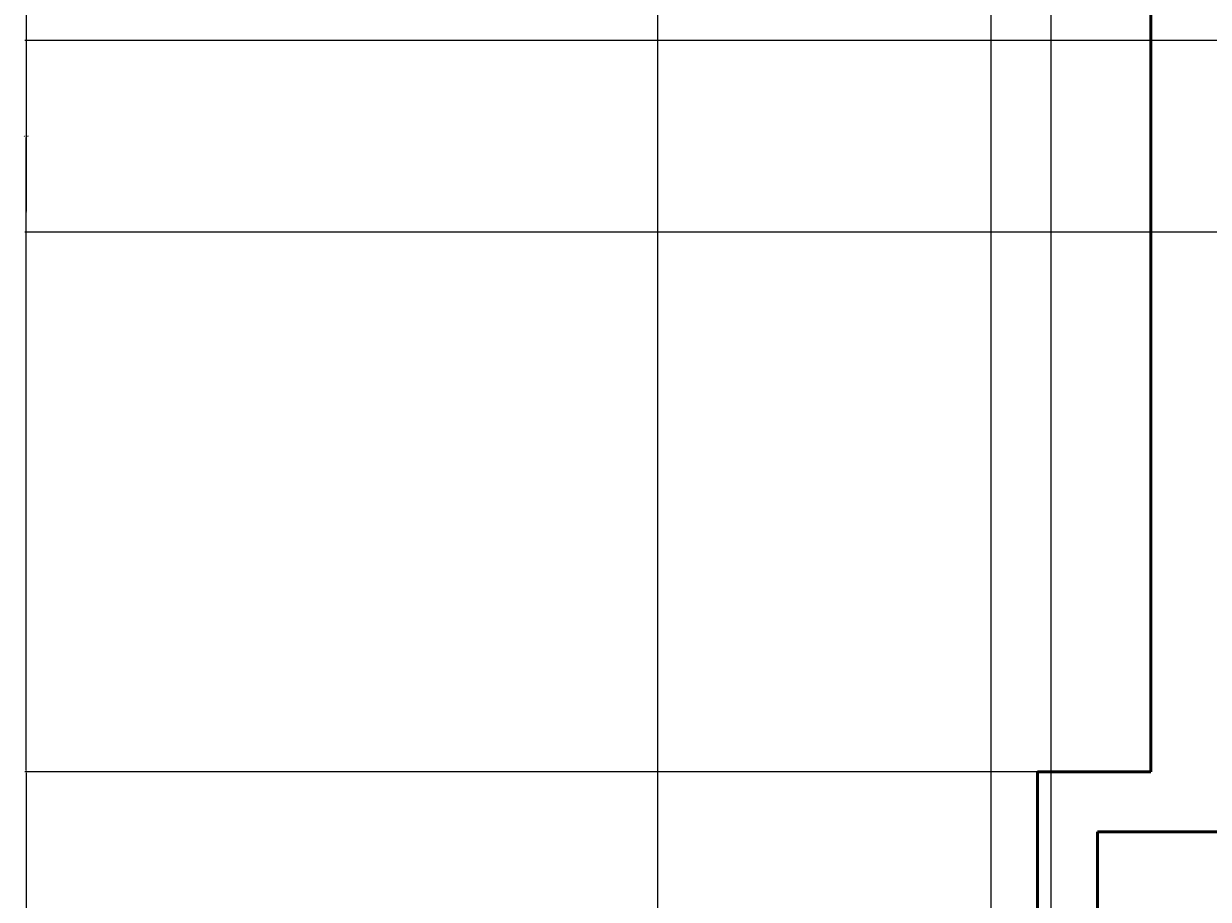
# Model space of a CAD drawing. Units: inches. Extents: x 5375 to 6084, y 16106 to 17259.
# Tile 18 of 32: x 5375 to 5553, y 16680 to 16812. Entities that reach past the tile are written whole.
import ezdxf

# ---------------------------------------------------------------- set-up
doc = ezdxf.new("R2010")
doc.units = ezdxf.units.IN
doc.layers.add('A-ANNO-DIMS', color=2, linetype='Continuous', lineweight=18)
doc.layers.add('WALL', color=6, linetype='Continuous', lineweight=50)
doc.styles.get("Standard").update_dxf_attribs({"font": 'arial.ttf'})
doc.dimstyles.get("Standard").update_dxf_attribs({"dimtxt": 0.18, "dimasz": 0.18, "dimexe": 0.18, "dimexo": 0.0625, "dimgap": 0.09, "dimtad": 0, "dimtih": 1, "dimtoh": 1, "dimdec": 4, "dimzin": 0, "dimdsep": 46, "dimtxsty": 'Standard', "dimcen": 0.09, "dimadec": 0, "dimazin": 0, "dimtfac": 1, "dimtdec": 4, "dimtofl": 0, "dimtmove": 0, "dimatfit": 3, "dimfxl": 1, "dimtolj": 1, "dimtzin": 0, "dimarcsym": 0})

# ---------------------------------------------------------------- blocks, each defined once
blk = doc.blocks.new('*D35')
at = {"layer": 'A-ANNO-DIMS', "color": 0, "lineweight": -2, "transparency": 16777216}
for p, q in [((5527.56, 16699.58), (5375.56, 16699.58)), ((5375.74, 16699.4), (5375.74, 16651.76)), ((5375.74, 16603.76), (5375.74, 16651.4)), ((5527.56, 16603.58), (5375.56, 16603.58))]:
    blk.add_line(p, q, dxfattribs=at)
at = {"layer": 'A-ANNO-DIMS', "color": 0, "transparency": 16777216}
for points in [[(5375.71, 16699.4), (5375.77, 16699.4), (5375.74, 16699.58)], [(5375.71, 16603.76), (5375.77, 16603.76), (5375.74, 16603.58)]]:
    blk.add_solid(points, dxfattribs=at)
at = {"layer": 'Defpoints', "color": 0, "transparency": 16777216}
for p in [(5375.74, 16699.58), (5527.62, 16699.58), (5527.62, 16603.58)]:
    blk.add_point(p, dxfattribs=at)
at = {"layer": 'A-ANNO-DIMS', "color": 0, "transparency": 16777216, "insert": (5375.74, 16651.58), "char_height": 0.18, "attachment_point": 5}
blk.add_mtext('\\A1;96', dxfattribs=at)
blk = doc.blocks.new('*D36')
at = {"layer": 'A-ANNO-DIMS', "color": 0, "lineweight": -2, "transparency": 16777216}
for p, q in [((5544.56, 16867.58), (5375.56, 16867.58)), ((5375.74, 16867.4), (5375.74, 16783.76)), ((5375.74, 16699.76), (5375.74, 16783.4)), ((5544.56, 16699.58), (5375.56, 16699.58))]:
    blk.add_line(p, q, dxfattribs=at)
at = {"layer": 'A-ANNO-DIMS', "color": 0, "transparency": 16777216}
for points in [[(5375.71, 16867.4), (5375.77, 16867.4), (5375.74, 16867.58)], [(5375.71, 16699.76), (5375.77, 16699.76), (5375.74, 16699.58)]]:
    blk.add_solid(points, dxfattribs=at)
at = {"layer": 'Defpoints', "color": 0, "transparency": 16777216}
for p in [(5375.74, 16867.58), (5544.62, 16867.58), (5544.62, 16699.58)]:
    blk.add_point(p, dxfattribs=at)
at = {"layer": 'A-ANNO-DIMS', "color": 0, "transparency": 16777216, "insert": (5375.74, 16783.58), "char_height": 0.18, "attachment_point": 5}
blk.add_mtext('\\A1;168', dxfattribs=at)
blk = doc.blocks.new('*D40')
at = {"layer": 'A-ANNO-DIMS', "color": 0, "lineweight": -2, "transparency": 16777216}
for p, q in [((5529.62, 16876.52), (5529.62, 16106.48)), ((5520.62, 16867.52), (5520.62, 16106.48)), ((5520.8, 16106.66), (5524.97, 16106.66)), ((5529.44, 16106.66), (5525.27, 16106.66))]:
    blk.add_line(p, q, dxfattribs=at)
at = {"layer": 'A-ANNO-DIMS', "color": 0, "transparency": 16777216}
for points in [[(5520.8, 16106.69), (5520.8, 16106.63), (5520.62, 16106.66)], [(5529.44, 16106.69), (5529.44, 16106.63), (5529.62, 16106.66)]]:
    blk.add_solid(points, dxfattribs=at)
at = {"layer": 'Defpoints', "color": 0, "transparency": 16777216}
for p in [(5529.62, 16876.58), (5520.62, 16867.58), (5529.62, 16106.66)]:
    blk.add_point(p, dxfattribs=at)
at = {"layer": 'A-ANNO-DIMS', "color": 0, "transparency": 16777216, "insert": (5525.12, 16106.66), "char_height": 0.18, "attachment_point": 5}
blk.add_mtext('\\A1;9', dxfattribs=at)
blk = doc.blocks.new('*D43')
at = {"layer": 'A-ANNO-DIMS', "color": 0, "lineweight": -2, "transparency": 16777216}
for p, q in [((5826.06, 16809.37), (5375.56, 16809.37)), ((5375.74, 16809.19), (5375.74, 16795.15)), ((5375.74, 16780.76), (5375.74, 16794.79)), ((5826.06, 16780.58), (5375.56, 16780.58))]:
    blk.add_line(p, q, dxfattribs=at)
at = {"layer": 'A-ANNO-DIMS', "color": 0, "transparency": 16777216}
for points in [[(5375.71, 16809.19), (5375.77, 16809.19), (5375.74, 16809.37)], [(5375.71, 16780.76), (5375.77, 16780.76), (5375.74, 16780.58)]]:
    blk.add_solid(points, dxfattribs=at)
at = {"layer": 'Defpoints', "color": 0, "transparency": 16777216}
for p in [(5375.74, 16809.37), (5826.12, 16809.37), (5826.12, 16780.58)]:
    blk.add_point(p, dxfattribs=at)
at = {"layer": 'A-ANNO-DIMS', "color": 0, "transparency": 16777216, "insert": (5375.74, 16794.97), "char_height": 0.18, "attachment_point": 5}
blk.add_mtext('\\A1;28.786', dxfattribs=at)
blk = doc.blocks.new('*D47')
at = {"layer": 'A-ANNO-DIMS', "color": 0, "lineweight": -2, "transparency": 16777216}
for p, q in [((5470.62, 16603.64), (5470.62, 17259.16)), ((5470.8, 17258.98), (5495.4, 17258.98)), ((5520.44, 17258.98), (5495.84, 17258.98)), ((5520.62, 17206.64), (5520.62, 17259.16))]:
    blk.add_line(p, q, dxfattribs=at)
at = {"layer": 'A-ANNO-DIMS', "color": 0, "transparency": 16777216}
for points in [[(5470.8, 17259.01), (5470.8, 17258.95), (5470.62, 17258.98)], [(5520.44, 17259.01), (5520.44, 17258.95), (5520.62, 17258.98)]]:
    blk.add_solid(points, dxfattribs=at)
at = {"layer": 'Defpoints', "color": 0, "transparency": 16777216}
for p in [(5520.62, 17258.98), (5520.62, 17206.58), (5470.62, 16603.58)]:
    blk.add_point(p, dxfattribs=at)
at = {"layer": 'A-ANNO-DIMS', "color": 0, "transparency": 16777216, "insert": (5495.62, 17258.98), "char_height": 0.18, "attachment_point": 5}
blk.add_mtext('\\A1;50', dxfattribs=at)

msp = doc.modelspace()

# ---------------------------------------------------------------- linework, layer by layer
at = {"layer": 'WALL'}
for p, q in [((5544.6199, 16867.5793), (5544.6199, 16699.5793)), ((5527.6199, 16699.5793), (5544.6199, 16699.5793)), ((5527.6199, 16699.5793), (5527.6199, 16603.5793)), ((5536.6199, 16690.5793), (5698.6199, 16690.5793)), ((5536.6199, 16690.5793), (5536.6199, 16558.5793))]:
    msp.add_line(p, q, dxfattribs=at)

# ---------------------------------------------------------------- dimensions: what is measured, and where the dimension line sits
at = {"layer": 'A-ANNO-DIMS'}
for base, p1, p2, picture, middle in [((5520.6199, 17258.9793), (5470.6199, 16603.5793), (5520.6199, 17206.5793), '*D47', (5495.6199, 17258.9793)), ((5529.6199, 16106.6631), (5520.6199, 16867.5793), (5529.6199, 16876.5793), '*D40', (5525.1199, 16106.6631))]:
    dim = msp.add_linear_dim(base=base, p1=p1, p2=p2, dimstyle='Standard', override={"dimdec": 0, "dimlfac": 1, "dimrnd": 0, "dimzin": 0, "dimdsep": 46, "dimlunit": 2}, dxfattribs=at)
    dim.commit()
    dim.dimension.update_dxf_attribs({"geometry": picture, "text_midpoint": middle})
for base, p1, p2, override, picture, middle in [((5375.7423, 16867.5793), (5544.6199, 16699.5793), (5544.6199, 16867.5793), {"dimdec": 0, "dimlfac": 1, "dimrnd": 0, "dimzin": 0, "dimdsep": 46, "dimlunit": 2}, '*D36', (5375.7423, 16783.5793)), ((5375.7423, 16809.3651), (5826.1199, 16780.5793), (5826.1199, 16809.3651), {"dimdec": 3, "dimlfac": 1, "dimrnd": 0, "dimzin": 0, "dimdsep": 46, "dimlunit": 2}, '*D43', (5375.7423, 16794.9722)), ((5375.7423, 16699.5793), (5527.6199, 16603.5793), (5527.6199, 16699.5793), {"dimdec": 0, "dimlfac": 1, "dimrnd": 0, "dimzin": 0, "dimdsep": 46, "dimlunit": 2}, '*D35', (5375.7423, 16651.5793))]:
    dim = msp.add_linear_dim(base=base, p1=p1, p2=p2, angle=90, dimstyle='Standard', override=override, dxfattribs=at)
    dim.commit()
    dim.dimension.update_dxf_attribs({"geometry": picture, "text_midpoint": middle})

doc.saveas('drawing.dxf')
